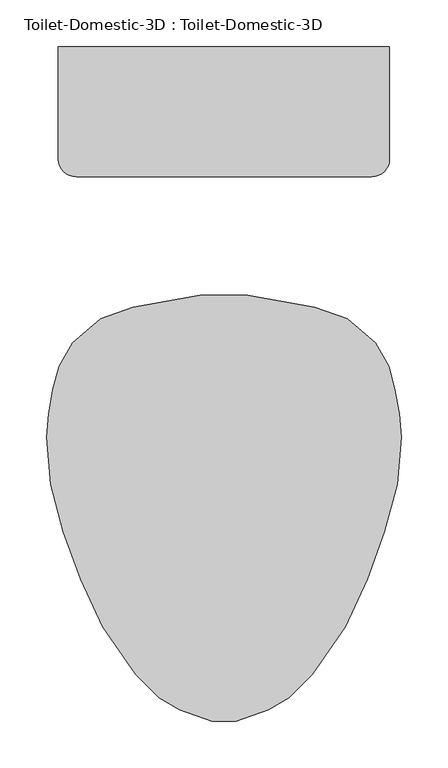
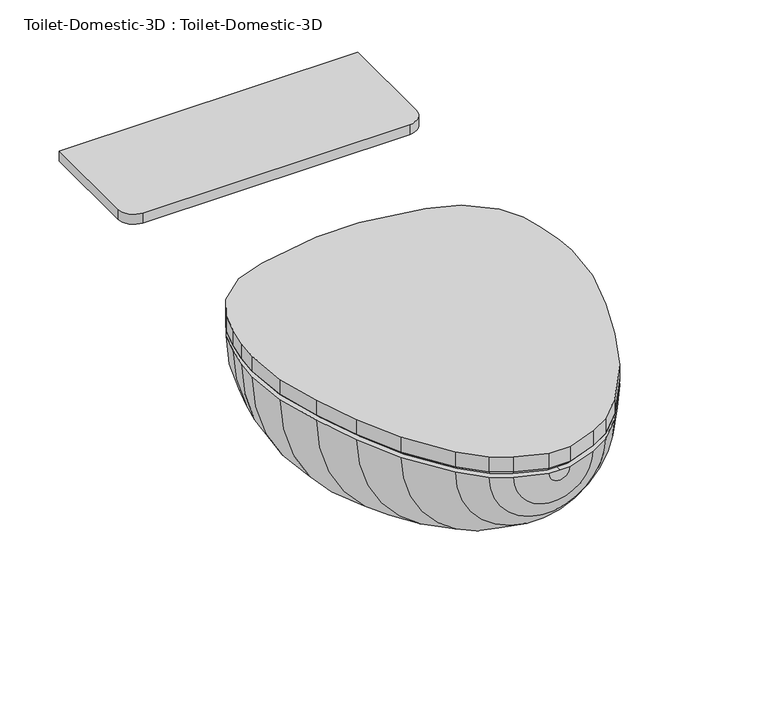
"""IFC4 building model written with IfcOpenShell, lengths in millimetres: flow terminal geometry, Toilet-Domestic-3D : Toilet-Domestic-3D."""

from ifc_helpers import new_model, si_unit, point, frame, frame_2d, origin, place, context, project, spatial, polyline, circle_curve, trimmed, segment, composite_curve, outline, extrude, faceted_brep, source, transform, mapped, element, save
from ifc_brep_helpers import plane_surface, revolved_surface, advanced_brep


def toilet_domestic_3d_toilet_domestic_3d_183bbd19(model_context):
    return source(origin(), model_context, "Body", "SolidModel", [
        advanced_brep(
        [(-25.4, 152.4, 361.95), (-97.4252791, 139.7, 361.95), (-132.3182423, 127.0, 361.95), (-162.5887836, 101.6, 361.95), (-176.9845865, 76.2, 361.95), (-183.790496, 50.8, 361.95), (-188.2862441, 25.3033453, 361.95), (-190.5, 0.0, 361.95), (-186.0724883, -50.6066907, 361.95), (-172.4088722, -101.6, 361.95), (-153.9191843, -152.4, 361.95), (-130.2307553, -203.2, 361.95), (-94.9900085, -254.0, 361.95), (-69.5900085, -279.4, 361.95), (-47.5929632, -292.1, 361.95), (-12.7, -304.8, 361.95), (0.0, -304.8, 361.95), (0.0, -284.592034, 361.95), (-12.5224565, -284.592034, 361.95), (-39.5113323, -274.7688865, 361.95), (-58.4178985, -263.8531754, 361.95), (-79.2146703, -243.0564036, 361.95), (-114.0255101, -192.8761202, 361.95), (-136.654021, -144.3491221, 361.95), (-154.575847, -95.1093097, 361.95), (-167.7238545, -46.0402777, 361.95), (-171.5645445, -2.1409906, 361.95), (-169.3087351, 23.6430284, 361.95), (-165.101298, 47.5045901, 361.95), (-159.5484355, 68.2281551, 361.95), (-146.1085923, 90.5605136, 361.95), (-121.9980886, 110.7916284, 361.95), (-94.1172813, 120.9394123, 361.95), (-22.0920022, 133.6394123, 361.95), (0.0, 133.6394123, 361.95), (0.0, 152.4, 361.95), (25.4, 152.4, 361.95), (22.0920022, 133.6394123, 361.95), (94.1172813, 120.9394123, 361.95), (121.9980886, 110.7916284, 361.95), (146.1085923, 90.5605136, 361.95), (159.5484355, 68.2281551, 361.95), (165.101298, 47.5045901, 361.95), (169.3087351, 23.6430284, 361.95), (171.5645445, -2.1409906, 361.95), (167.7238545, -46.0402777, 361.95), (154.575847, -95.1093097, 361.95), (136.654021, -144.3491221, 361.95), (114.0255101, -192.8761202, 361.95), (79.2146703, -243.0564036, 361.95), (58.4178985, -263.8531754, 361.95), (39.5113323, -274.7688865, 361.95), (12.5224565, -284.592034, 361.95), (12.7, -304.8, 361.95), (47.5929632, -292.1, 361.95), (69.5900085, -279.4, 361.95), (94.9900085, -254.0, 361.95), (130.2307553, -203.2, 361.95), (153.9191843, -152.4, 361.95), (172.4088722, -101.6, 361.95), (186.0724883, -50.6066907, 361.95), (190.5, 0.0, 361.95), (188.2862441, 25.3033453, 361.95), (183.790496, 50.8, 361.95), (176.9845865, 76.2, 361.95), (162.5887836, 101.6, 361.95), (132.3182423, 127.0, 361.95), (97.4252791, 139.7, 361.95)],
        [
            (0, 1),
            (1, 2),
            (2, 3),
            (3, 4),
            (4, 5),
            (5, 6),
            (6, 7),
            (7, 8),
            (8, 9),
            (9, 10),
            (10, 11),
            (11, 12),
            (12, 13),
            (13, 14),
            (14, 15),
            (15, 16),
            (16, 17),
            (17, 18),
            (18, 19),
            (19, 20),
            (20, 21),
            (21, 22),
            (22, 23),
            (23, 24),
            (24, 25),
            (25, 26),
            (26, 27),
            (27, 28),
            (28, 29),
            (29, 30),
            (30, 31),
            (31, 32),
            (32, 33),
            (33, 34),
            (34, 35),
            (35, 0),
            (36, 35),
            (34, 37),
            (37, 38),
            (38, 39),
            (39, 40),
            (40, 41),
            (41, 42),
            (42, 43),
            (43, 44),
            (44, 45),
            (45, 46),
            (46, 47),
            (47, 48),
            (48, 49),
            (49, 50),
            (50, 51),
            (51, 52),
            (52, 17),
            (16, 53),
            (53, 54),
            (54, 55),
            (55, 56),
            (56, 57),
            (57, 58),
            (58, 59),
            (59, 60),
            (60, 61),
            (61, 62),
            (62, 63),
            (63, 64),
            (64, 65),
            (65, 66),
            (66, 67),
            (67, 36),
            (67, 1, circle_curve(frame((0.0, 139.7, 361.95), z_axis=(0.0, 1.0, 0.0), x_axis=(-1.0, 0.0, 0.0)), 97.4252791)),
            (0, 36, circle_curve(frame((0.0, 152.4, 361.95), z_axis=(0.0, -1.0, 0.0), x_axis=(-1.0, 0.0, 0.0)), 25.4)),
            (66, 2, circle_curve(frame((0.0, 127.0, 361.95), z_axis=(0.0, 1.0, 0.0), x_axis=(-1.0, 0.0, 0.0)), 132.3182423)),
            (65, 3, circle_curve(frame((0.0, 101.6, 361.95), z_axis=(0.0, 1.0, 0.0), x_axis=(-1.0, 0.0, 0.0)), 162.5887836)),
            (64, 4, circle_curve(frame((0.0, 76.2, 361.95), z_axis=(0.0, 1.0, 0.0), x_axis=(-1.0, 0.0, 0.0)), 176.9845865)),
            (63, 5, circle_curve(frame((0.0, 50.8, 361.95), z_axis=(0.0, 1.0, 0.0), x_axis=(-1.0, 0.0, 0.0)), 183.790496)),
            (62, 6, circle_curve(frame((0.0, 25.3033453, 361.95), z_axis=(0.0, 1.0, 0.0), x_axis=(-1.0, 0.0, 0.0)), 188.2862441)),
            (61, 7, circle_curve(frame((0.0, 0.0, 361.95), z_axis=(0.0, 1.0, 0.0), x_axis=(-1.0, 0.0, 0.0)), 190.5)),
            (60, 8, circle_curve(frame((0.0, -50.6066907, 361.95), z_axis=(0.0, 1.0, 0.0), x_axis=(-1.0, 0.0, 0.0)), 186.0724883)),
            (59, 9, circle_curve(frame((0.0, -101.6, 361.95), z_axis=(0.0, 1.0, 0.0), x_axis=(-1.0, 0.0, 0.0)), 172.4088722)),
            (58, 10, circle_curve(frame((0.0, -152.4, 361.95), z_axis=(0.0, 1.0, 0.0), x_axis=(-1.0, 0.0, 0.0)), 153.9191843)),
            (57, 11, circle_curve(frame((0.0, -203.2, 361.95), z_axis=(0.0, 1.0, 0.0), x_axis=(-1.0, 0.0, 0.0)), 130.2307553)),
            (56, 12, circle_curve(frame((0.0, -254.0, 361.95), z_axis=(0.0, 1.0, 0.0), x_axis=(-1.0, 0.0, 0.0)), 94.9900085)),
            (55, 13, circle_curve(frame((0.0, -279.4, 361.95), z_axis=(0.0, 1.0, 0.0), x_axis=(-1.0, 0.0, 0.0)), 69.5900085)),
            (54, 14, circle_curve(frame((0.0, -292.1, 361.95), z_axis=(0.0, 1.0, 0.0), x_axis=(-1.0, 0.0, 0.0)), 47.5929632)),
            (53, 15, circle_curve(frame((0.0, -304.8, 361.95), z_axis=(0.0, 1.0, 0.0), x_axis=(-1.0, 0.0, 0.0)), 12.7)),
            (52, 18, circle_curve(frame((0.0, -284.592034, 361.95), z_axis=(0.0, 1.0, 0.0), x_axis=(-1.0, 0.0, 0.0)), 12.5224565)),
            (51, 19, circle_curve(frame((0.0, -274.7688865, 361.95), z_axis=(0.0, 1.0, 0.0), x_axis=(-1.0, 0.0, 0.0)), 39.5113323)),
            (50, 20, circle_curve(frame((0.0, -263.8531754, 361.95), z_axis=(0.0, 1.0, 0.0), x_axis=(-1.0, 0.0, 0.0)), 58.4178985)),
            (49, 21, circle_curve(frame((0.0, -243.0564036, 361.95), z_axis=(0.0, 1.0, 0.0), x_axis=(-1.0, 0.0, 0.0)), 79.2146703)),
            (48, 22, circle_curve(frame((0.0, -192.8761202, 361.95), z_axis=(0.0, 1.0, 0.0), x_axis=(-1.0, 0.0, 0.0)), 114.0255101)),
            (47, 23, circle_curve(frame((0.0, -144.3491221, 361.95), z_axis=(0.0, 1.0, 0.0), x_axis=(-1.0, 0.0, 0.0)), 136.654021)),
            (46, 24, circle_curve(frame((0.0, -95.1093097, 361.95), z_axis=(0.0, 1.0, 0.0), x_axis=(-1.0, 0.0, 0.0)), 154.575847)),
            (45, 25, circle_curve(frame((0.0, -46.0402777, 361.95), z_axis=(0.0, 1.0, 0.0), x_axis=(-1.0, 0.0, 0.0)), 167.7238545)),
            (44, 26, circle_curve(frame((0.0, -2.1409906, 361.95), z_axis=(0.0, 1.0, 0.0), x_axis=(-1.0, 0.0, 0.0)), 171.5645445)),
            (43, 27, circle_curve(frame((0.0, 23.6430284, 361.95), z_axis=(0.0, 1.0, 0.0), x_axis=(-1.0, 0.0, 0.0)), 169.3087351)),
            (42, 28, circle_curve(frame((0.0, 47.5045901, 361.95), z_axis=(0.0, 1.0, 0.0), x_axis=(-1.0, 0.0, 0.0)), 165.101298)),
            (41, 29, circle_curve(frame((0.0, 68.2281551, 361.95), z_axis=(0.0, 1.0, 0.0), x_axis=(-1.0, 0.0, 0.0)), 159.5484355)),
            (40, 30, circle_curve(frame((0.0, 90.5605136, 361.95), z_axis=(0.0, 1.0, 0.0), x_axis=(-1.0, 0.0, 0.0)), 146.1085923)),
            (39, 31, circle_curve(frame((0.0, 110.7916284, 361.95), z_axis=(0.0, 1.0, 0.0), x_axis=(-1.0, 0.0, 0.0)), 121.9980886)),
            (38, 32, circle_curve(frame((0.0, 120.9394123, 361.95), z_axis=(0.0, 1.0, 0.0), x_axis=(-1.0, 0.0, 0.0)), 94.1172813)),
            (37, 33, circle_curve(frame((0.0, 133.6394123, 361.95), z_axis=(0.0, 1.0, 0.0), x_axis=(-1.0, 0.0, 0.0)), 22.0920022)),
        ],
        [
            plane_surface(frame((0.0, 175.1599017, 361.95), z_axis=(0.0, 0.0, 1.0), x_axis=(-1.0, 0.0, 0.0))),
            plane_surface(frame((0.0, 175.1599017, 361.95), z_axis=(0.0, 0.0, 1.0), x_axis=(1.0, 0.0, 0.0))),
            revolved_surface(polyline([(-25.4, 152.4, 361.95), (-97.4252791, 139.7, 361.95)]), (0.0, 175.1599017, 361.95), (0.0, -1.0, 0.0)),
            revolved_surface(polyline([(-97.4252791, 139.7, 361.95), (-132.3182423, 127.0, 361.95)]), (0.0, 175.1599017, 361.95), (0.0, -1.0, 0.0)),
            revolved_surface(polyline([(-132.3182423, 127.0, 361.95), (-162.5887836, 101.6, 361.95)]), (0.0, 175.1599017, 361.95), (0.0, -1.0, 0.0)),
            revolved_surface(polyline([(-162.5887836, 101.6, 361.95), (-176.9845865, 76.2, 361.95)]), (0.0, 175.1599017, 361.95), (0.0, -1.0, 0.0)),
            revolved_surface(polyline([(-176.9845865, 76.2, 361.95), (-183.790496, 50.8, 361.95)]), (0.0, 175.1599017, 361.95), (0.0, -1.0, 0.0)),
            revolved_surface(polyline([(-183.790496, 50.8, 361.95), (-188.2862441, 25.3033453, 361.95)]), (0.0, 175.1599017, 361.95), (0.0, -1.0, 0.0)),
            revolved_surface(polyline([(-188.2862441, 25.3033453, 361.95), (-190.5, 0.0, 361.95)]), (0.0, 175.1599017, 361.95), (0.0, -1.0, 0.0)),
            revolved_surface(polyline([(-190.5, 0.0, 361.95), (-186.0724883, -50.6066907, 361.95)]), (0.0, 175.1599017, 361.95), (0.0, -1.0, 0.0)),
            revolved_surface(polyline([(-186.0724883, -50.6066907, 361.95), (-172.4088722, -101.6, 361.95)]), (0.0, 175.1599017, 361.95), (0.0, -1.0, 0.0)),
            revolved_surface(polyline([(-172.4088722, -101.6, 361.95), (-153.9191843, -152.4, 361.95)]), (0.0, 175.1599017, 361.95), (0.0, -1.0, 0.0)),
            revolved_surface(polyline([(-153.9191843, -152.4, 361.95), (-130.2307553, -203.2, 361.95)]), (0.0, 175.1599017, 361.95), (0.0, -1.0, 0.0)),
            revolved_surface(polyline([(-130.2307553, -203.2, 361.95), (-94.9900085, -254.0, 361.95)]), (0.0, 175.1599017, 361.95), (0.0, -1.0, 0.0)),
            revolved_surface(polyline([(-94.9900085, -254.0, 361.95), (-69.5900085, -279.4, 361.95)]), (0.0, 175.1599017, 361.95), (0.0, -1.0, 0.0)),
            revolved_surface(polyline([(-69.5900085, -279.4, 361.95), (-47.5929632, -292.1, 361.95)]), (0.0, 175.1599017, 361.95), (0.0, -1.0, 0.0)),
            revolved_surface(polyline([(-47.5929632, -292.1, 361.95), (-12.7, -304.8, 361.95)]), (0.0, 175.1599017, 361.95), (0.0, -1.0, 0.0)),
            plane_surface(frame((0.0, -304.8, 361.95), z_axis=(0.0, -1.0, 0.0), x_axis=(-1.0, 0.0, 0.0))),
            plane_surface(frame((0.0, -284.592034, 361.95), z_axis=(0.0, 1.0, 0.0), x_axis=(-1.0, 0.0, 0.0))),
            revolved_surface(polyline([(-12.5224565, -284.592034, 361.95), (-39.5113323, -274.7688865, 361.95)]), (0.0, 175.1599017, 361.95), (0.0, -1.0, 0.0)),
            revolved_surface(polyline([(-39.5113323, -274.7688865, 361.95), (-58.4178985, -263.8531754, 361.95)]), (0.0, 175.1599017, 361.95), (0.0, -1.0, 0.0)),
            revolved_surface(polyline([(-58.4178985, -263.8531754, 361.95), (-79.2146703, -243.0564036, 361.95)]), (0.0, 175.1599017, 361.95), (0.0, -1.0, 0.0)),
            revolved_surface(polyline([(-79.2146703, -243.0564036, 361.95), (-114.0255101, -192.8761202, 361.95)]), (0.0, 175.1599017, 361.95), (0.0, -1.0, 0.0)),
            revolved_surface(polyline([(-114.0255101, -192.8761202, 361.95), (-136.654021, -144.3491221, 361.95)]), (0.0, 175.1599017, 361.95), (0.0, -1.0, 0.0)),
            revolved_surface(polyline([(-136.654021, -144.3491221, 361.95), (-154.575847, -95.1093097, 361.95)]), (0.0, 175.1599017, 361.95), (0.0, -1.0, 0.0)),
            revolved_surface(polyline([(-154.575847, -95.1093097, 361.95), (-167.7238545, -46.0402777, 361.95)]), (0.0, 175.1599017, 361.95), (0.0, -1.0, 0.0)),
            revolved_surface(polyline([(-167.7238545, -46.0402777, 361.95), (-171.5645445, -2.1409906, 361.95)]), (0.0, 175.1599017, 361.95), (0.0, -1.0, 0.0)),
            revolved_surface(polyline([(-171.5645445, -2.1409906, 361.95), (-169.3087351, 23.6430284, 361.95)]), (0.0, 175.1599017, 361.95), (0.0, -1.0, 0.0)),
            revolved_surface(polyline([(-169.3087351, 23.6430284, 361.95), (-165.101298, 47.5045901, 361.95)]), (0.0, 175.1599017, 361.95), (0.0, -1.0, 0.0)),
            revolved_surface(polyline([(-165.101298, 47.5045901, 361.95), (-159.5484355, 68.2281551, 361.95)]), (0.0, 175.1599017, 361.95), (0.0, -1.0, 0.0)),
            revolved_surface(polyline([(-159.5484355, 68.2281551, 361.95), (-146.1085923, 90.5605136, 361.95)]), (0.0, 175.1599017, 361.95), (0.0, -1.0, 0.0)),
            revolved_surface(polyline([(-146.1085923, 90.5605136, 361.95), (-121.9980886, 110.7916284, 361.95)]), (0.0, 175.1599017, 361.95), (0.0, -1.0, 0.0)),
            revolved_surface(polyline([(-121.9980886, 110.7916284, 361.95), (-94.1172813, 120.9394123, 361.95)]), (0.0, 175.1599017, 361.95), (0.0, -1.0, 0.0)),
            revolved_surface(polyline([(-94.1172813, 120.9394123, 361.95), (-22.0920022, 133.6394123, 361.95)]), (0.0, 175.1599017, 361.95), (0.0, -1.0, 0.0)),
            plane_surface(frame((0.0, 133.6394123, 361.95), z_axis=(0.0, -1.0, 0.0), x_axis=(-1.0, 0.0, 0.0))),
            plane_surface(frame((0.0, 152.4, 361.95), z_axis=(0.0, 1.0, 0.0), x_axis=(-1.0, 0.0, 0.0))),
        ],
        [
            (0, [[1, 2, 3, 4, 5, 6, 7, 8, 9, 10, 11, 12, 13, 14, 15, 16, 17, 18, 19, 20, 21, 22, 23, 24, 25, 26, 27, 28, 29, 30, 31, 32, 33, 34, 35, 36]]),
            (1, [[37, -35, 38, 39, 40, 41, 42, 43, 44, 45, 46, 47, 48, 49, 50, 51, 52, 53, 54, -17, 55, 56, 57, 58, 59, 60, 61, 62, 63, 64, 65, 66, 67, 68, 69, 70]]),
            (2, [[71, -1, 72, -70]]),
            (3, [[73, -2, -71, -69]]),
            (4, [[74, -3, -73, -68]]),
            (5, [[75, -4, -74, -67]]),
            (6, [[76, -5, -75, -66]]),
            (7, [[77, -6, -76, -65]]),
            (8, [[78, -7, -77, -64]]),
            (9, [[79, -8, -78, -63]]),
            (10, [[80, -9, -79, -62]]),
            (11, [[81, -10, -80, -61]]),
            (12, [[82, -11, -81, -60]]),
            (13, [[83, -12, -82, -59]]),
            (14, [[84, -13, -83, -58]]),
            (15, [[85, -14, -84, -57]]),
            (16, [[86, -15, -85, -56]]),
            (17, [[-16, -86, -55]]),
            (18, [[87, -18, -54]]),
            (19, [[88, -19, -87, -53]]),
            (20, [[89, -20, -88, -52]]),
            (21, [[90, -21, -89, -51]]),
            (22, [[91, -22, -90, -50]]),
            (23, [[92, -23, -91, -49]]),
            (24, [[93, -24, -92, -48]]),
            (25, [[94, -25, -93, -47]]),
            (26, [[95, -26, -94, -46]]),
            (27, [[96, -27, -95, -45]]),
            (28, [[97, -28, -96, -44]]),
            (29, [[98, -29, -97, -43]]),
            (30, [[99, -30, -98, -42]]),
            (31, [[100, -31, -99, -41]]),
            (32, [[101, -32, -100, -40]]),
            (33, [[102, -33, -101, -39]]),
            (34, [[-34, -102, -38]]),
            (35, [[-72, -36, -37]]),
        ],
    ),
        faceted_brep([(-97.4252791, 139.7, 368.3), (-132.3182423, 127.0, 368.3), (-162.5887836, 101.6, 368.3), (-176.9845865, 76.2, 368.3), (-183.790496, 50.8, 368.3), (-188.2862441, 25.3033453, 368.3), (-190.5, 0.0, 368.3), (-186.0724883, -50.6066907, 368.3), (-172.4088722, -101.6, 368.3), (-153.9191843, -152.4, 368.3), (-130.2307553, -203.2, 368.3), (-94.9900085, -254.0, 368.3), (-69.5900085, -279.4, 368.3), (-47.5929632, -292.1, 368.3), (-12.7, -304.8, 368.3), (12.7, -304.8, 368.3), (47.5929632, -292.1, 368.3), (69.5900085, -279.4, 368.3), (94.9900085, -254.0, 368.3), (130.2307553, -203.2, 368.3), (153.9191843, -152.4, 368.3), (172.4088722, -101.6, 368.3), (186.0724883, -50.6066907, 368.3), (190.5, 0.0, 368.3), (188.2862441, 25.3033453, 368.3), (183.790496, 50.8, 368.3), (176.9845865, 76.2, 368.3), (162.5887836, 101.6, 368.3), (132.3182423, 127.0, 368.3), (97.4252791, 139.7, 368.3), (25.4, 152.4, 368.3), (-25.4, 152.4, 368.3), (-95.7755003, 133.5429415, 361.95), (-24.844447, 146.05, 361.95), (24.844447, 146.05, 361.95), (95.7755003, 133.5429415, 361.95), (129.0942628, 121.4159037, 361.95), (157.6293435, 97.472128, 361.95), (171.060664, 73.773864, 361.95), (177.5851102, 49.4242991, 361.95), (181.9845715, 24.4737144, 361.95), (184.125744, 0.0, 361.95), (179.7950716, -49.4998127, 361.95), (166.347, -99.688699, 361.95), (148.0469602, -149.9676451, 361.95), (124.7045808, -200.0255393, 361.95), (90.0971582, -249.9125941, 361.95), (65.691017, -274.3187354, 361.95), (44.8990862, -286.3229622, 361.95), (11.5803237, -298.45, 361.95), (-11.5803237, -298.45, 361.95), (-44.8990862, -286.3229622, 361.95), (-65.691017, -274.3187354, 361.95), (-90.0971582, -249.9125941, 361.95), (-124.7045808, -200.0255393, 361.95), (-148.0469602, -149.9676451, 361.95), (-166.347, -99.688699, 361.95), (-179.7950716, -49.4998127, 361.95), (-184.125744, 0.0, 361.95), (-181.9845715, 24.4737144, 361.95), (-177.5851102, 49.4242991, 361.95), (-171.060664, 73.773864, 361.95), (-157.6293435, 97.472128, 361.95), (-129.0942628, 121.4159037, 361.95)], [[[0, 1, 2, 3, 4, 5, 6, 7, 8, 9, 10, 11, 12, 13, 14, 15, 16, 17, 18, 19, 20, 21, 22, 23, 24, 25, 26, 27, 28, 29, 30, 31]], [[32, 33, 34, 35, 36, 37, 38, 39, 40, 41, 42, 43, 44, 45, 46, 47, 48, 49, 50, 51, 52, 53, 54, 55, 56, 57, 58, 59, 60, 61, 62, 63]], [[32, 63, 1, 0]], [[63, 62, 2, 1]], [[62, 61, 3, 2]], [[61, 60, 4, 3]], [[60, 59, 5, 4]], [[59, 58, 6, 5]], [[58, 57, 7, 6]], [[57, 56, 8, 7]], [[56, 55, 9, 8]], [[55, 54, 10, 9]], [[54, 53, 11, 10]], [[53, 52, 12, 11]], [[52, 51, 13, 12]], [[51, 50, 14, 13]], [[50, 49, 15, 14]], [[49, 48, 16, 15]], [[48, 47, 17, 16]], [[47, 46, 18, 17]], [[46, 45, 19, 18]], [[45, 44, 20, 19]], [[44, 43, 21, 20]], [[43, 42, 22, 21]], [[42, 41, 23, 22]], [[41, 40, 24, 23]], [[40, 39, 25, 24]], [[39, 38, 26, 25]], [[38, 37, 27, 26]], [[37, 36, 28, 27]], [[36, 35, 29, 28]], [[35, 34, 30, 29]], [[34, 33, 31, 30]], [[33, 32, 0, 31]]]),
        extrude(outline(composite_curve([segment(polyline([(177.8, 419.1), (177.8, 298.45)]), True, "CONTINUOUS"), segment(trimmed(circle_curve(frame_2d((158.75, 298.45)), 19.05), [point((177.8, 298.45))], [point((158.75, 279.4))], False, "CARTESIAN"), True, "CONTINUOUS"), segment(polyline([(158.75, 279.4), (-158.75, 279.4)]), True, "CONTINUOUS"), segment(trimmed(circle_curve(frame_2d((-158.75, 298.45)), 19.05), [point((-158.75, 279.4))], [point((-177.8, 298.45))], False, "CARTESIAN"), True, "CONTINUOUS"), segment(polyline([(-177.8, 298.45), (-177.8, 419.1), (177.8, 419.1)]), True, "CONTINUOUS")], self_intersect=False)), frame((0.0, 0.0, 374.65), z_axis=(0.0, 0.0, 1.0), x_axis=(1.0, 0.0, 0.0)), (0.0, 0.0, 1.0), 12.5681453),
        extrude(outline(polyline([(-162.5887836, 101.6), (-132.3182423, 127.0), (-97.4252791, 139.7), (-25.4, 152.4), (25.4, 152.4), (97.4252791, 139.7), (132.3182423, 127.0), (162.5887836, 101.6), (176.9845865, 76.2), (183.790496, 50.8), (188.2862441, 25.3033453), (190.5, 0.0), (186.0724883, -50.6066907), (172.4088722, -101.6), (153.9191843, -152.4), (130.2307553, -203.2), (94.9900085, -254.0), (69.5900085, -279.4), (47.5929632, -292.1), (12.7, -304.8), (-12.7, -304.8), (-47.5929632, -292.1), (-69.5900085, -279.4), (-94.9900085, -254.0), (-130.2307553, -203.2), (-153.9191843, -152.4), (-172.4088722, -101.6), (-186.0724883, -50.6066907), (-190.5, 0.0), (-188.2862441, 25.3033453), (-183.790496, 50.8), (-176.9845865, 76.2), (-162.5887836, 101.6)])), frame((0.0, 0.0, 368.3), z_axis=(0.0, 0.0, 1.0), x_axis=(1.0, 0.0, 0.0)), (0.0, 0.0, 1.0), 19.05),
    ])


if __name__ == "__main__":
    model = new_model("IFC4")
    model_context = context("Model", 3, world=origin())
    ifc_project = project(units=[si_unit("LENGTHUNIT", "METRE", prefix="MILLI")], contexts=[model_context])
    site = spatial("IfcSite", under=ifc_project)
    building = spatial("IfcBuilding", under=site)
    placement = place(None, origin())
    toilet_domestic_3d_toilet_domestic_3d_shape = toilet_domestic_3d_toilet_domestic_3d_183bbd19(model_context)
    element("IfcFlowTerminal", 1, ObjectType="Toilet-Domestic-3D : Toilet-Domestic-3D", at=placement, inside=building, context=model_context, shape_type="MappedRepresentation", body=[
        mapped(toilet_domestic_3d_toilet_domestic_3d_shape, transform((0.0, 0.0, 0.0), x_axis=(1.0, 0.0, 0.0), y_axis=(0.0, 1.0, 0.0), z_axis=(0.0, 0.0, 1.0))),
    ])
    save(model, "model.ifc")

# Revit data of these elements
# Type "Toilet-Domestic-3D : Toilet-Domestic-3D"
#   Assembly Code = "D2010110"
#   Toilet - Bowl/Basin Material = Porcelain, Linen
#   Toilet - Seat Material = Laminate, Linen, Matte
# Element 1 (IfcFlowTerminal, "Toilet-Domestic-3D : Toilet-Domestic-3D")
#   Materials on its faces: "Porcelain, Linen", "Laminate, Linen, Matte"
# Materials
#   "Porcelain, Linen": class "Ceramic", colour RGB 249 239 230, transparency 0, Description = "Porcelain, linen", Cost = 0
#   "Laminate, Linen, Matte": class "Plastic", colour RGB 249 239 230, transparency 0, Description = "Plastic Laminate - Linen, Matte", Cost = 0
